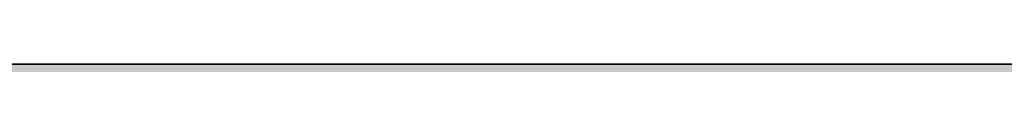
# Model space of a CAD drawing. Units: inches. Extents: x 2091 to 2899, y 967 to 2217.
# Tile 80 of 256: x 2223.2 to 2238.36, y 1099.92 to 1099.92. Entities that reach past the tile are written whole.
import ezdxf

# ---------------------------------------------------------------- set-up
doc = ezdxf.new("R2010")
doc.units = ezdxf.units.IN
doc.layers.add('A-WALL-PATT', color=141, linetype='Continuous', lineweight=13, true_color=0xadddf7)
doc.layers.add('L-SITE-WALL', color=7, linetype='Continuous', lineweight=35)

msp = doc.modelspace()

# ---------------------------------------------------------------- hatches: boundary and pattern name
at = {"layer": 'A-WALL-PATT'}
h = msp.add_hatch(color=256, dxfattribs=at)
h.dxf.hatch_style = 1
h.paths.add_polyline_path([(2212.144, 1941.419), (2387.644, 1941.419), (2387.644, 1824.419), (2392.144, 1824.419), (2392.144, 1941.419), (2609.644, 1941.419), (2609.644, 1825.919), (2614.144, 1825.919), (2614.144, 1941.419), (2794.144, 1941.419), (2794.144, 1928.762), (2803.144, 1928.762), (2803.144, 2050.919), (2203.144, 2050.919), (2203.144, 1900.758), (2212.144, 1900.758)])
h.paths.add_polyline_path([(2212.144, 1945.919), (2212.144, 2041.919), (2794.144, 2041.919), (2794.144, 1945.919), (2402.248, 1945.919), (2401.102, 1945.776), (2398.702, 1945.776)], flags=16)
h.paths.add_polyline_path([(2230.23, 1948.063), (2227.35, 1949.503), (2225.91, 1951.903), (2223.99, 1952.863), (2223.03, 1955.263), (2222.07, 1959.583), (2222.07, 1963.423), (2223.03, 1965.663), (2223.99, 1965.343), (2225.586, 1963.861), (2226.912, 1964.957), (2226.949, 1965.939), (2227.778, 1966.952), (2228.2, 1968.879), (2230.71, 1964.863), (2233.59, 1966.303), (2233.607, 1966.332), (2233.773, 1964.938), (2234.634, 1963.676), (2235.03, 1963.903), (2236.282, 1965.572), (2235.99, 1962.943), (2237.955, 1957.54), (2238.39, 1957.903), (2239.216, 1960.306), (2238.655, 1966.385), (2238.693, 1966.438), (2238.841, 1967.5), (2238.78, 1967.687), (2238.881, 1967.787), (2238.667, 1966.252), (2239.216, 1960.306), (2238.39, 1957.903), (2236.95, 1956.703), (2234.55, 1949.983)], flags=0)
h.paths.add_polyline_path([(2278.012, 1948.063), (2276.496, 1947.873), (2275.85, 1947.689), (2274.652, 1947.103)], flags=0)
h.paths.add_polyline_path([(2269.852, 1955.743), (2268.276, 1956.629), (2270.867, 1956.348), (2269.372, 1958.143), (2268.715, 1959.192), (2270.57, 1958.729), (2268.581, 1961.906), (2270.812, 1960.892), (2270.812, 1963.423), (2271.393, 1964.779), (2270.292, 1966.156), (2271.772, 1965.663), (2272.141, 1966.525), (2273.93, 1965.929), (2275.63, 1968.054), (2276.332, 1966.722), (2276.52, 1966.952), (2276.942, 1968.879), (2277.734, 1967.611), (2278.14, 1969.465), (2279.659, 1967.034), (2280.412, 1966.783), (2280.949, 1967.589), (2281.61, 1967.369), (2282.133, 1968.154), (2282.349, 1966.333), (2282.35, 1966.333), (2283.408, 1968.095), (2283.713, 1965.524), (2284.32, 1964.634), (2284.512, 1964.889), (2284.235, 1965.705), (2284.5, 1967.319), (2284.908, 1965.417), (2285.396, 1966.069), (2285.433, 1966.291), (2285.473, 1966.171), (2286.354, 1967.345), (2286.222, 1966.158), (2287.663, 1968.08), (2287.714, 1968.443), (2288.482, 1969.017), (2288.574, 1968.729), (2288.917, 1969.069), (2288.607, 1966.838), (2288.929, 1963.351), (2288.935, 1963.357), (2288.93, 1963.34), (2289.015, 1962.414), (2290.111, 1963.875), (2290.133, 1963.943), (2290.218, 1964.017), (2290.111, 1963.875), (2289.156, 1960.892), (2288.594, 1959.257), (2288.572, 1959.103), (2289.532, 1960.543), (2290.012, 1962.463), (2290.192, 1962.643), (2289.77, 1959.689), (2286.89, 1957.289), (2284.49, 1950.569), (2283.315, 1950.046), (2283.292, 1949.983), (2280.29, 1948.649), (2281.13, 1948.649), (2282.57, 1948.169), (2283.205, 1948.063), (2278.972, 1948.063), (2276.092, 1949.503), (2274.652, 1951.903), (2272.732, 1952.863)], flags=0)
h.paths.add_polyline_path([(2271.159, 1958.022), (2272.97, 1955.849), (2272.01, 1960.169), (2272.01, 1964.009), (2272.624, 1965.443), (2274.328, 1963.861), (2275.654, 1964.957), (2275.638, 1964.539), (2277.412, 1966.007), (2277.033, 1965.157), (2276.83, 1964.976), (2276.766, 1963.295), (2277.45, 1962.66), (2279.452, 1964.863), (2282.332, 1966.303), (2283.53, 1966.889), (2283.295, 1966.771), (2283.913, 1963.885), (2284.899, 1964.448), (2284.732, 1962.943), (2286.697, 1957.54), (2287.132, 1957.903), (2287.542, 1959.095), (2287.779, 1958.442), (2285.683, 1956.695), (2285.877, 1959.795), (2284.732, 1962.943), (2284.899, 1964.448), (2283.913, 1963.885), (2284.224, 1962.434), (2283.424, 1963.605), (2281.61, 1962.569), (2281.13, 1960.169), (2282.09, 1956.329), (2283.05, 1952.969), (2282.57, 1950.569), (2280.17, 1948.649), (2279.883, 1948.792), (2278.972, 1948.063), (2278.972, 1949.023), (2278.672, 1949.397), (2277.29, 1950.089), (2275.85, 1952.489), (2273.93, 1953.449), (2272.49, 1954.889), (2271.922, 1954.889), (2271.772, 1955.263)], flags=0)
h.paths.add_polyline_path([(2311.994, 1955.743), (2312.063, 1955.674), (2312.055, 1955.709)], flags=0)
h.paths.add_polyline_path([(2331.956, 1963.952), (2333.396, 1965.392), (2331.077, 1963.357), (2330.999, 1963.112)], flags=0)
h.paths.add_polyline_path([(2310.554, 1954.303), (2307.04, 1956.28), (2310.763, 1955.876), (2312.474, 1953.823), (2313.434, 1951.423), (2315.354, 1950.463), (2316.794, 1948.063), (2317.466, 1947.727), (2319.369, 1947.965), (2317.754, 1949.983), (2317.57, 1950.61), (2316.794, 1951.903), (2314.874, 1952.863), (2313.914, 1955.263), (2311.514, 1958.143), (2309.375, 1961.559), (2311.514, 1960.337), (2311.514, 1961.983), (2310.605, 1963.12), (2311.727, 1962.479), (2312.418, 1964.093), (2312.256, 1964.296), (2313.194, 1963.983), (2313.914, 1965.663), (2314.647, 1965.419), (2315.354, 1966.303), (2316.794, 1967.743), (2316.157, 1966.947), (2317.034, 1965.282), (2317.223, 1965.512), (2317.777, 1968.046), (2318.474, 1966.722), (2318.663, 1966.952), (2319.084, 1968.879), (2321.207, 1965.482), (2322.161, 1966.914), (2322.554, 1966.783), (2322.786, 1967.131), (2322.882, 1966.324), (2323.312, 1965.722), (2323.651, 1965.891), (2324.396, 1967.133), (2324.657, 1964.938), (2324.972, 1964.477), (2325.387, 1967.001), (2325.941, 1964.418), (2327.229, 1966.136), (2327.166, 1965.572), (2328.059, 1966.763), (2328.225, 1966.247), (2329.668, 1967.677), (2329.665, 1967.687), (2329.765, 1967.787), (2329.551, 1966.252), (2330.1, 1960.306), (2329.333, 1958.073), (2329.313, 1957.935), (2329.634, 1958.203), (2330.234, 1959.103), (2330.714, 1961.023), (2331.034, 1961.343), (2330.714, 1959.103), (2329.634, 1958.203), (2329.274, 1957.663), (2327.712, 1956.361), (2325.434, 1949.983), (2324.334, 1949.494), (2323.994, 1948.543), (2319.674, 1946.623), (2316.794, 1948.063), (2315.354, 1950.463), (2313.434, 1951.423)], flags=0)
h.paths.add_polyline_path([(2321.336, 1947.952), (2321.114, 1948.063), (2321.114, 1949.023), (2319.194, 1951.423), (2316.794, 1959.583), (2316.663, 1959.583), (2315.354, 1958.143), (2314.394, 1958.143), (2313.148, 1958.709), (2312.954, 1959.583), (2312.954, 1960.892), (2315.834, 1959.583), (2316.663, 1959.583), (2317.315, 1960.299), (2315.03, 1962.421), (2316.356, 1963.517), (2316.372, 1963.952), (2316.47, 1963.861), (2317.796, 1964.957), (2317.755, 1963.89), (2319.175, 1965.157), (2319.498, 1965.881), (2321.114, 1965.343), (2323.236, 1962.372), (2325.686, 1963.773), (2325.543, 1962.481), (2325.199, 1963.494), (2324.479, 1963.082), (2324.926, 1960.994), (2324.078, 1962.236), (2322.415, 1961.286), (2322.074, 1959.583), (2323.034, 1955.743), (2323.994, 1952.383), (2323.514, 1949.983), (2322.143, 1948.886), (2322.074, 1948.543)], flags=0)
h.paths.add_polyline_path([(2320.207, 1963.337), (2320.154, 1963.423), (2320.394, 1963.543)], flags=0)
h.paths.add_polyline_path([(2353.851, 1965.811), (2354.031, 1965.751), (2354.331, 1966.451), (2354.331, 1966.931)], flags=0)
h.paths.add_polyline_path([(2359.021, 1969.026), (2359.098, 1968.902), (2359.234, 1969.52), (2359.234, 1970)], flags=0)
h.paths.add_polyline_path([(2358.257, 1966.682), (2357.984, 1966.348), (2358.211, 1966.146), (2358.41, 1966.39)], flags=0)
h.paths.add_polyline_path([(2357.768, 1966.059), (2357.732, 1965.105), (2357.751, 1965.121), (2357.77, 1965.607), (2357.77, 1966.058)], flags=0)
h.paths.add_polyline_path([(2359.112, 1965.305), (2359.112, 1964.825), (2359.845, 1966.468), (2359.845, 1966.948)], flags=0)
h.paths.add_polyline_path([(2360.224, 1966.621), (2360.699, 1969.363), (2360.699, 1969.843), (2360.211, 1967.026), (2360.211, 1966.643)], flags=0)
h.paths.add_polyline_path([(2363.451, 1967.891), (2363.451, 1968.371), (2362.491, 1966.931), (2362.656, 1966.699)], flags=0)
h.paths.add_polyline_path([(2364.476, 1966.079), (2365.851, 1968.371), (2365.851, 1968.851), (2364.428, 1966.48)], flags=0)
h.paths.add_polyline_path([(2366.314, 1965.853), (2366.367, 1965.696), (2366.803, 1968.346), (2366.803, 1968.826)], flags=0)
h.paths.add_polyline_path([(2367.165, 1965.804), (2367.291, 1966.931), (2367.291, 1967.411), (2367.103, 1965.72)], flags=0)
h.paths.add_polyline_path([(2370.037, 1959.974), (2371.014, 1963.025), (2371.014, 1963.505), (2370.037, 1960.454)], flags=0)
h.paths.add_polyline_path([(2371.611, 1960.211), (2372.571, 1961.651), (2372.571, 1962.131), (2371.803, 1960.979)], flags=0)
h.paths.add_polyline_path([(2350.874, 1956.005), (2351.931, 1955.891), (2354.491, 1953.331), (2353.851, 1954.931), (2351.451, 1957.811), (2347.936, 1963.426), (2347.936, 1963.906), (2351.451, 1958.291), (2353.705, 1955.585), (2352.891, 1959.251), (2352.891, 1959.731), (2352.891, 1961.925), (2356.731, 1959.731), (2358.454, 1961.627), (2354.811, 1965.011), (2355.031, 1965.286), (2358.691, 1961.887), (2361.531, 1965.011), (2364.376, 1966.433), (2364.524, 1965.187), (2365.454, 1963.824), (2365.881, 1964.068), (2365.371, 1966.451), (2365.371, 1966.931), (2366.811, 1960.211), (2366.811, 1959.731), (2366.389, 1952.981), (2367.771, 1956.851), (2368.641, 1957.576), (2366.811, 1962.611), (2366.811, 1963.091), (2368.775, 1957.688), (2369.211, 1958.051), (2370.002, 1960.352), (2369.475, 1966.053), (2369.513, 1966.106), (2369.514, 1966.111), (2369.475, 1966.533), (2369.513, 1966.586), (2369.615, 1967.313), (2369.183, 1968.659), (2369.183, 1969.139), (2369.601, 1967.835), (2369.701, 1967.934), (2369.718, 1968.055), (2370.145, 1968.374), (2369.779, 1968.011), (2369.701, 1967.454), (2370.468, 1968.214), (2369.675, 1967.266), (2369.514, 1966.111), (2370.037, 1960.454), (2370.037, 1959.974), (2369.442, 1958.243), (2370.651, 1959.251), (2371.046, 1962.018), (2371.131, 1962.131), (2370.651, 1958.771), (2367.771, 1956.371), (2365.371, 1949.651), (2362.079, 1948.188), (2363.451, 1947.731), (2361.051, 1947.731), (2360.091, 1947.731), (2357.104, 1947.357), (2360.091, 1948.211), (2358.171, 1949.171), (2356.731, 1951.571), (2354.811, 1952.531), (2351.931, 1955.411)], flags=0)
h.paths.add_polyline_path([(2361.051, 1948.691), (2359.131, 1951.091), (2356.731, 1959.251), (2355.771, 1959.251), (2352.891, 1960.56), (2352.891, 1961.445), (2355.891, 1959.731), (2356.731, 1959.731), (2356.837, 1959.368), (2361.531, 1964.531), (2363.248, 1965.389), (2364.925, 1963.042), (2362.491, 1961.651), (2362.064, 1959.517), (2362.971, 1955.891), (2363.931, 1952.531), (2363.931, 1952.051), (2363.451, 1949.651), (2361.051, 1947.731)], flags=0)
h.paths.add_polyline_path([(2359.131, 1951.571), (2359.291, 1951.371), (2361.051, 1954.451), (2361.051, 1954.931)], flags=0)
h.paths.add_polyline_path([(2357.22, 1966.546), (2356.793, 1968.815), (2356.793, 1969.295), (2357.22, 1967.026)], flags=0)
h.paths.add_polyline_path([(2361.051, 1954.451), (2361.531, 1958.771), (2361.531, 1959.251), (2361.051, 1954.931)], flags=0)
h.paths.add_polyline_path([(2402.548, 1948.486), (2402.302, 1948.416), (2402.59, 1948.416)], flags=0)
h.paths.add_polyline_path([(2394.142, 1956.096), (2395.685, 1954.553), (2396.72, 1953.971), (2396.062, 1955.616), (2395.241, 1956.601), (2395.879, 1956.442), (2395.102, 1959.936), (2395.102, 1963.776), (2396.062, 1966.016), (2397.022, 1965.696), (2398.618, 1964.214), (2399.944, 1965.31), (2399.981, 1966.292), (2400.811, 1967.305), (2401.232, 1969.232), (2403.538, 1965.543), (2403.942, 1967.389), (2404.702, 1967.136), (2405.46, 1966.075), (2406.622, 1966.656), (2406.64, 1966.685), (2406.805, 1965.291), (2406.926, 1965.115), (2407.342, 1964.976), (2407.874, 1965.774), (2408.169, 1964.398), (2409.315, 1965.925), (2409.217, 1965.051), (2409.445, 1963.131), (2410.306, 1961.87), (2410.702, 1962.096), (2411.442, 1963.082), (2411.165, 1963.898), (2411.616, 1966.64), (2411.725, 1966.791), (2411.873, 1967.853), (2411.813, 1968.041), (2411.913, 1968.14), (2411.699, 1966.605), (2412.248, 1960.659), (2413.225, 1963.71), (2414.378, 1964.721), (2414.513, 1965.693), (2414.453, 1965.881), (2414.553, 1965.98), (2414.378, 1964.721), (2414.52, 1964.846), (2414.365, 1964.631), (2414.339, 1964.445), (2414.888, 1958.499), (2414.062, 1956.096), (2412.622, 1954.896), (2410.171, 1948.033), (2410.017, 1948.084), (2405.902, 1946.256), (2405.902, 1947.216), (2405.204, 1948.089), (2404.222, 1948.416), (2403.262, 1948.416), (2400.382, 1949.856), (2399.662, 1951.056), (2397.982, 1952.736), (2397.022, 1953.216), (2395.685, 1954.553), (2392.657, 1956.257)], flags=0)
h.paths.add_polyline_path([(2409.086, 1964.407), (2409.13, 1964.276), (2409.262, 1964.496)], flags=0)
h.paths.add_polyline_path([(2397.742, 1961.616), (2398.702, 1963.856), (2399.662, 1963.536), (2401.427, 1965.741), (2401.791, 1966.559), (2402.071, 1965.071), (2402.836, 1964.393), (2403.262, 1964.915), (2403.338, 1964.771), (2402.616, 1963.976), (2402.499, 1960.902), (2403.543, 1959.932), (2404.413, 1960.89), (2404.702, 1962.336), (2407.916, 1964.172), (2409.52, 1961.927), (2410.987, 1957.893), (2411.422, 1958.256), (2412.048, 1960.076), (2412.41, 1959.079), (2411.676, 1958.467), (2411.662, 1958.256), (2411.626, 1958.426), (2409.982, 1957.056), (2407.582, 1950.336), (2403.262, 1948.416), (2403.262, 1949.376), (2401.342, 1951.776), (2399.417, 1958.324), (2397.742, 1959.085), (2397.742, 1959.97), (2397.102, 1960.336), (2397.742, 1960.045)], flags=0)
h.paths.add_polyline_path([(2405.902, 1952.976), (2405.95, 1953.408), (2406.017, 1953.176)], flags=0)
h.paths.add_polyline_path([(2449.818, 1967.114), (2449.752, 1967.136), (2449.794, 1967.078)], flags=0)
h.paths.add_polyline_path([(2451.698, 1966.618), (2451.741, 1966.69), (2451.692, 1966.666)], flags=0)
h.paths.add_polyline_path([(2454.344, 1965.738), (2455.752, 1967.616), (2455.992, 1968.096), (2454.364, 1965.925)], flags=0)
h.paths.add_polyline_path([(2457.547, 1968.864), (2457.787, 1969.344), (2457.054, 1968.796), (2457.008, 1968.46)], flags=0)
h.paths.add_polyline_path([(2456.922, 1967.857), (2456.802, 1968.229), (2456.723, 1967.66)], flags=0)
h.paths.add_polyline_path([(2457.302, 1967.377), (2457.542, 1967.857), (2456.81, 1966.84), (2456.741, 1966.7), (2456.749, 1966.608)], flags=0)
h.paths.add_polyline_path([(2458.275, 1963.71), (2458.155, 1963.335), (2460.354, 1965.265), (2460.594, 1965.745)], flags=0)
h.paths.add_polyline_path([(2458.392, 1962.816), (2458.364, 1962.618), (2459.592, 1964.256), (2459.832, 1964.736)], flags=0)
h.paths.add_polyline_path([(2459.352, 1962.816), (2459.272, 1962.496), (2460.072, 1963.296), (2460.312, 1963.776)], flags=0)
h.paths.add_polyline_path([(2458.68, 1960.608), (2458.632, 1960.416), (2459.592, 1961.856), (2459.832, 1962.336)], flags=0)
h.paths.add_polyline_path([(2437.838, 1956.243), (2439.192, 1956.096), (2441.352, 1953.936), (2440.872, 1955.136), (2438.472, 1958.016), (2438.072, 1958.656), (2438.712, 1958.496), (2440.64, 1956.183), (2439.912, 1959.456), (2439.912, 1963.296), (2441.352, 1966.656), (2441.592, 1967.136), (2441.112, 1966.016), (2442.072, 1965.696), (2443.989, 1968.092), (2444.241, 1966.751), (2444.917, 1966.152), (2445.677, 1967.08), (2446.255, 1969.725), (2446.495, 1970.205), (2446.282, 1969.232), (2447.363, 1967.503), (2447.72, 1969.568), (2447.96, 1970.048), (2447.485, 1967.307), (2448.792, 1965.216), (2448.472, 1964.864), (2448.552, 1964.736), (2451.452, 1966.186), (2451.615, 1964.811), (2452.308, 1963.796), (2453.235, 1964.326), (2454.072, 1960.416), (2453.629, 1953.318), (2454.792, 1956.576), (2455.032, 1957.056), (2455.719, 1957.628), (2453.832, 1962.816), (2453.941, 1963.794), (2453.335, 1965.578), (2453.824, 1968.551), (2454.064, 1969.031), (2453.575, 1966.058), (2454.04, 1964.688), (2453.832, 1962.816), (2455.719, 1957.628), (2456.367, 1958.168), (2457.058, 1960.179), (2457.298, 1960.659), (2456.472, 1958.256), (2457.718, 1959.294), (2457.672, 1958.976), (2454.89, 1956.657), (2453.614, 1953.085), (2453.592, 1952.736), (2453.352, 1952.256), (2453.36, 1952.372), (2452.632, 1950.336), (2452.392, 1949.856), (2449.204, 1948.439), (2450.712, 1947.936), (2448.072, 1947.936), (2447.112, 1947.936), (2444.552, 1947.616), (2447.2, 1948.372), (2445.192, 1949.376), (2443.752, 1951.776), (2441.832, 1952.736), (2438.952, 1955.616)], flags=0)
h.paths.add_polyline_path([(2443.992, 1959.936), (2444.04, 1959.773), (2444.122, 1959.862)], flags=0)
h.paths.add_polyline_path([(2442.912, 1959.936), (2443.032, 1959.936), (2442.446, 1960.202)], flags=0)
h.paths.add_polyline_path([(2444.983, 1965.02), (2445.279, 1965.265), (2445.519, 1965.745), (2444.994, 1965.31)], flags=0)
h.paths.add_polyline_path([(2446.133, 1965.03), (2446.33, 1965.471), (2444.97, 1964.258), (2444.73, 1963.778)], flags=0)
h.paths.add_polyline_path([(2442.792, 1959.456), (2443.752, 1959.456), (2446.152, 1951.296), (2446.412, 1951.751), (2446.392, 1951.776), (2448.081, 1954.73), (2448.552, 1958.976), (2441.832, 1965.216), (2442.155, 1965.619), (2448.792, 1959.456), (2448.312, 1955.136), (2448.072, 1954.656), (2446.412, 1951.751), (2448.312, 1949.376), (2448.312, 1948.416), (2450.541, 1950.199), (2450.952, 1952.256), (2449.992, 1955.616), (2449.032, 1959.456), (2449.512, 1961.856), (2449.752, 1962.336), (2449.675, 1961.949), (2452.995, 1963.846), (2453.064, 1963.519), (2452.885, 1963.783), (2449.675, 1961.949), (2449.272, 1959.936), (2450.232, 1956.096), (2451.192, 1952.736), (2450.712, 1950.336), (2450.472, 1949.856), (2448.072, 1947.936), (2448.072, 1948.536), (2445.432, 1949.856), (2443.992, 1952.256), (2442.072, 1953.216), (2441.112, 1955.616), (2440.152, 1959.936), (2440.152, 1960.656)], flags=0)
h.paths.add_polyline_path([(2456.692, 1966.986), (2457.608, 1968.081), (2457.848, 1968.561), (2456.932, 1967.466)], flags=0)
h.paths.add_polyline_path([(2489.897, 1966.58), (2489.943, 1966.189), (2490.747, 1967.53), (2491.319, 1968.951)], flags=0)
h.paths.add_polyline_path([(2473.562, 1956.407), (2477.14, 1956.019), (2476.955, 1956.241), (2475.108, 1957.28), (2476.347, 1956.97), (2475.187, 1958.824), (2476.919, 1958.391), (2475.412, 1960.799), (2477.787, 1959.719), (2477.787, 1962.25), (2477.637, 1962.438), (2477.823, 1962.332), (2478.359, 1963.584), (2478.359, 1963.671), (2477.324, 1964.965), (2478.715, 1964.501), (2479.319, 1965.911), (2480.279, 1965.591), (2481.784, 1967.472), (2482.116, 1965.705), (2482.881, 1965.028), (2483.209, 1965.429), (2483.22, 1965.715), (2483.076, 1965.989), (2483.712, 1966.766), (2484.13, 1968.679), (2484.702, 1970.1), (2484.489, 1969.127), (2486.503, 1965.905), (2487.387, 1965.61), (2488.153, 1966.759), (2488.717, 1965.97), (2489.2, 1966.212), (2489.331, 1965.111), (2490.394, 1963.622), (2490.661, 1963.775), (2490.494, 1964.554), (2490.923, 1963.925), (2491.319, 1964.151), (2491.333, 1964.17), (2491.21, 1964.532), (2491.282, 1964.966), (2491.426, 1964.293), (2494.076, 1967.828), (2494.498, 1966.515), (2494.598, 1966.614), (2494.689, 1967.27), (2495.107, 1967.582), (2495.13, 1967.748), (2495.07, 1967.936), (2495.17, 1968.035), (2495.032, 1967.044), (2495.754, 1967.759), (2494.982, 1966.686), (2494.956, 1966.5), (2495.479, 1960.837), (2495.91, 1962.184), (2496.482, 1963.605), (2496.073, 1962.327), (2496.769, 1962.938), (2496.599, 1962.711), (2496.119, 1959.351), (2496.733, 1960.272), (2496.987, 1961.29), (2497.559, 1962.711), (2497.079, 1960.791), (2496.507, 1959.37), (2495.547, 1957.93), (2492.759, 1955.606), (2490.839, 1950.231), (2490.267, 1948.81), (2485.947, 1946.89), (2483.067, 1948.33), (2481.627, 1950.73), (2479.707, 1951.69), (2476.827, 1954.57)], flags=0)
h.paths.add_polyline_path([(2485.577, 1948.313), (2485.559, 1948.311), (2485.579, 1948.311)], flags=0)
h.paths.add_polyline_path([(2478.645, 1954.551), (2478.109, 1956.963), (2479.319, 1955.511), (2480.279, 1953.111), (2482.199, 1952.151), (2483.639, 1949.751), (2486.519, 1948.311), (2486.519, 1949.271), (2484.739, 1951.496), (2484.027, 1950.25), (2481.627, 1958.41), (2482.375, 1959.233), (2482.199, 1959.831), (2483.198, 1960.929), (2479.707, 1964.17), (2480.603, 1965.29), (2481.875, 1964.109), (2482.666, 1964.764), (2482.615, 1963.422), (2482.989, 1963.075), (2484.008, 1963.984), (2484.684, 1965.498), (2484.58, 1965.405), (2485.357, 1967.147), (2485.121, 1965.781), (2486.427, 1963.69), (2488.145, 1964.549), (2489.822, 1962.202), (2490.747, 1962.73), (2492, 1964.4), (2492.076, 1965.087), (2492.213, 1964.684), (2492.485, 1965.047), (2492.279, 1963.191), (2494.244, 1957.788), (2494.563, 1958.054), (2494.933, 1959.133), (2495.505, 1960.554), (2494.679, 1958.151), (2494.107, 1956.73), (2494.563, 1958.054), (2493.409, 1957.092), (2491.707, 1961.77), (2492, 1964.4), (2490.747, 1962.73), (2487.712, 1960.996), (2487.479, 1959.831), (2488.439, 1955.991), (2489.399, 1952.631), (2488.919, 1950.231), (2488.577, 1949.957), (2488.347, 1948.81), (2487.652, 1948.254), (2487.479, 1948.311), (2486.519, 1948.311), (2483.639, 1949.751), (2482.199, 1952.151), (2480.279, 1953.111), (2478.839, 1954.551)], flags=0)
h.paths.add_polyline_path([(2526.648, 1966.988), (2526.517, 1967.031), (2526.6, 1966.915)], flags=0)
h.paths.add_polyline_path([(2528.471, 1966.447), (2528.574, 1966.62), (2528.457, 1966.561)], flags=0)
h.paths.add_polyline_path([(2534.133, 1967.496), (2534.157, 1967.543), (2534.06, 1967.408)], flags=0)
h.paths.add_polyline_path([(2536.162, 1964.051), (2535.157, 1962.711), (2535.101, 1962.316), (2536.117, 1963.671), (2536.421, 1964.278)], flags=0)
h.paths.add_polyline_path([(2535.157, 1959.831), (2536.117, 1961.271), (2536.597, 1962.231), (2535.253, 1960.215)], flags=0)
h.paths.add_polyline_path([(2513.249, 1956.285), (2516.221, 1955.963), (2514.997, 1957.431), (2514.196, 1958.712), (2515.477, 1958.391), (2516.932, 1956.646), (2516.437, 1958.871), (2516.437, 1962.711), (2516.873, 1963.727), (2515.346, 1965.635), (2517.397, 1964.951), (2517.877, 1966.071), (2518.357, 1967.031), (2517.877, 1965.911), (2518.837, 1965.591), (2520.487, 1967.653), (2520.766, 1966.166), (2521.53, 1965.489), (2521.781, 1965.795), (2521.801, 1966.307), (2521.478, 1966.921), (2521.246, 1967.126), (2521.178, 1967.491), (2521.478, 1966.921), (2522.01, 1966.449), (2522.257, 1966.75), (2522.78, 1969.14), (2523.26, 1970.1), (2523.047, 1969.127), (2524.673, 1966.526), (2526.037, 1966.071), (2526.795, 1965.01), (2527.977, 1965.601), (2528.14, 1964.227), (2528.665, 1963.458), (2529.389, 1963.872), (2529.33, 1964.147), (2529.481, 1963.925), (2529.877, 1964.151), (2529.984, 1964.293), (2529.789, 1965.203), (2530.062, 1964.398), (2532.802, 1968.051), (2533.148, 1966.976), (2533.248, 1967.075), (2533.339, 1967.731), (2533.673, 1967.98), (2533.728, 1968.035), (2533.514, 1966.5), (2534.025, 1960.972), (2534.56, 1962.645), (2535.04, 1963.605), (2534.063, 1960.554), (2533.237, 1958.151), (2534.288, 1959.027), (2534.197, 1958.391), (2531.513, 1956.154), (2529.397, 1950.231), (2528.917, 1949.271), (2526.449, 1948.174), (2527.477, 1947.831), (2530.357, 1947.351), (2524.597, 1947.351), (2521.717, 1948.791), (2520.277, 1951.191), (2518.357, 1952.151), (2515.477, 1955.031)], flags=0)
h.paths.add_polyline_path([(2523.935, 1967.19), (2523.62, 1966.484), (2523.77, 1966.242)], flags=0)
h.paths.add_polyline_path([(2518.837, 1953.111), (2517.877, 1955.511), (2516.885, 1959.977), (2516.917, 1959.962), (2516.917, 1962.025), (2520.757, 1959.831), (2522.025, 1961.226), (2518.357, 1964.631), (2519.003, 1965.438), (2520.433, 1964.109), (2521.301, 1964.827), (2521.245, 1963.355), (2525.638, 1959.276), (2526.037, 1961.271), (2529.397, 1963.191), (2530.65, 1964.861), (2530.665, 1964.998), (2530.692, 1964.917), (2531.088, 1965.445), (2530.946, 1964.169), (2530.692, 1964.917), (2529.397, 1963.191), (2526.363, 1961.457), (2526.037, 1959.831), (2526.997, 1955.991), (2527.957, 1952.631), (2527.477, 1950.231), (2527.134, 1949.957), (2526.974, 1949.154), (2526.697, 1949.031), (2524.597, 1947.351), (2524.597, 1948.311), (2524.277, 1948.711), (2522.197, 1949.751), (2520.757, 1952.151)], flags=0)
h.paths.add_polyline_path([(2520.277, 1958.871), (2520.853, 1959.505), (2523.157, 1951.671), (2524.614, 1954.22), (2524.597, 1954.071), (2522.677, 1950.711)], flags=0)
h.paths.add_polyline_path([(2559.371, 1966.311), (2559.398, 1966.325), (2559.402, 1966.345)], flags=0)
h.paths.add_polyline_path([(2549.771, 1957.191), (2552.651, 1954.311), (2552.134, 1955.603), (2550.611, 1957.431), (2547.096, 1963.046), (2545.776, 1965.206), (2549.291, 1959.591), (2551.691, 1956.711), (2550.793, 1960.752), (2550.731, 1960.78), (2550.731, 1964.871), (2551.691, 1967.111), (2552.651, 1966.791), (2554.247, 1965.309), (2555.034, 1965.96), (2555.582, 1966.645), (2555.61, 1967.387), (2556.439, 1968.401), (2556.861, 1970.327), (2559.371, 1966.311), (2560.691, 1964.151), (2562.409, 1965.01), (2561.651, 1966.071), (2560.331, 1968.231), (2561.758, 1966.233), (2562.347, 1967.116), (2562.434, 1966.387), (2563.128, 1965.37), (2563.571, 1965.591), (2563.588, 1965.62), (2563.363, 1967.524), (2563.722, 1965.844), (2565.06, 1968.073), (2564.733, 1965.129), (2565.118, 1963.333), (2567.445, 1966.436), (2567.316, 1967.833), (2567.354, 1967.886), (2567.502, 1968.948), (2567.441, 1969.136), (2567.542, 1969.235), (2567.328, 1967.7), (2567.877, 1961.754), (2568.747, 1964.47), (2568.636, 1965.673), (2568.674, 1965.726), (2568.822, 1966.788), (2568.761, 1966.976), (2568.862, 1967.075), (2568.648, 1965.54), (2568.726, 1964.693), (2568.854, 1964.805), (2568.747, 1964.47), (2568.817, 1963.706), (2568.971, 1963.911), (2568.866, 1963.177), (2569.197, 1959.594), (2568.371, 1957.191), (2566.931, 1955.991), (2564.62, 1949.521), (2564.651, 1949.511), (2564.617, 1949.511), (2564.531, 1949.271), (2560.211, 1947.351), (2557.331, 1948.791), (2556.045, 1950.934), (2556.011, 1950.951), (2555.857, 1951.208), (2553.971, 1952.151), (2551.091, 1955.031), (2546.65, 1957.53)], flags=0)
h.paths.add_polyline_path([(2567.026, 1959.33), (2567.035, 1959.305), (2567.051, 1959.351)], flags=0)
h.paths.add_polyline_path([(2551.968, 1962.518), (2553.011, 1964.951), (2553.971, 1964.631), (2555.567, 1963.149), (2556.893, 1964.246), (2556.93, 1965.227), (2557.144, 1965.489), (2556.42, 1966.131), (2556.391, 1966.105), (2556.38, 1966.166), (2556.42, 1966.131), (2556.952, 1966.605), (2557.092, 1966.919), (2557.571, 1966.01), (2557.759, 1966.241), (2557.418, 1964.68), (2556.893, 1964.246), (2556.807, 1961.998), (2560.691, 1958.391), (2560.636, 1957.893), (2560.811, 1957.191), (2561.771, 1953.831), (2561.291, 1951.431), (2559.11, 1949.687), (2559.156, 1949.629), (2563.027, 1951.349), (2562.611, 1949.271), (2560.211, 1947.351), (2560.211, 1948.311), (2559.251, 1949.511), (2558.891, 1949.511), (2558.891, 1949.961), (2558.291, 1950.711), (2558.054, 1951.518), (2556.971, 1952.871), (2555.068, 1959.341), (2552.051, 1961.065), (2552.051, 1962.471)], flags=0)
h.paths.add_polyline_path([(2588.33, 1958.391), (2588.61, 1958.111), (2588.553, 1958.367)], flags=0)
h.paths.add_polyline_path([(2594.745, 1950.493), (2593.958, 1953.172), (2593.13, 1954.551), (2591.21, 1955.511), (2590.25, 1957.911), (2588.309, 1960.24), (2586.177, 1961.209), (2587.85, 1960.791), (2587.253, 1961.744), (2588.441, 1961.065), (2588.441, 1962.656), (2588.422, 1962.665), (2588.441, 1962.711), (2586.914, 1964.62), (2588.877, 1963.728), (2589.29, 1964.692), (2589.29, 1966.071), (2590.25, 1968.311), (2591.21, 1967.991), (2592.806, 1966.509), (2594.132, 1967.606), (2594.169, 1968.587), (2594.999, 1969.601), (2595.42, 1971.527), (2597.93, 1967.511), (2600.81, 1968.951), (2600.827, 1968.98), (2600.993, 1967.587), (2601.854, 1966.325), (2602.107, 1966.47), (2602.236, 1967.255), (2602.357, 1966.693), (2603.502, 1968.221), (2603.21, 1965.591), (2605.175, 1960.188), (2605.507, 1960.465), (2605.026, 1965.673), (2605.064, 1965.726), (2605.212, 1966.788), (2605.152, 1966.976), (2605.252, 1967.075), (2605.343, 1967.731), (2605.953, 1968.187), (2605.875, 1969.033), (2605.913, 1969.086), (2606.061, 1970.148), (2606, 1970.336), (2606.101, 1970.435), (2605.887, 1968.9), (2606.436, 1962.954), (2605.61, 1960.551), (2605.997, 1960.874), (2606.564, 1962.645), (2608.241, 1964.117), (2608.01, 1963.191), (2607.05, 1961.751), (2606.631, 1961.402), (2606.201, 1958.391), (2603.321, 1955.991), (2600.921, 1949.271), (2596.601, 1947.351), (2593.721, 1948.791), (2592.857, 1950.231), (2592.65, 1950.231)], flags=0)
h.paths.add_polyline_path([(2596.601, 1947.351), (2596.601, 1948.311), (2594.681, 1950.711), (2596.155, 1953.29), (2595.53, 1954.071), (2593.199, 1961.996), (2592.651, 1962.505), (2591.78, 1963.003), (2593.283, 1964.246), (2593.32, 1965.227), (2594.15, 1966.241), (2594.571, 1968.167), (2596.183, 1965.589), (2596.951, 1966.435), (2598.041, 1966.071), (2598.799, 1965.01), (2599.961, 1965.591), (2599.979, 1965.62), (2600.144, 1964.227), (2601.005, 1962.965), (2601.401, 1963.191), (2602.653, 1964.861), (2602.361, 1962.231), (2603.793, 1958.295), (2601.978, 1953.212), (2601.946, 1952.709), (2599.469, 1951.608), (2599.001, 1949.271)], flags=0)
h.paths.add_polyline_path([(2597.561, 1958.871), (2597.671, 1959.419), (2597.595, 1958.736)], flags=0)
h.paths.add_polyline_path([(2623.666, 1961.254), (2625.519, 1960.791), (2624.966, 1961.676), (2627.199, 1960.66), (2627.199, 1961.151), (2626.959, 1962.231), (2626.959, 1963.491), (2625.582, 1965.212), (2626.959, 1964.425), (2626.959, 1965.831), (2626.869, 1965.861), (2627.919, 1968.311), (2628.879, 1967.991), (2630.475, 1966.509), (2631.801, 1967.606), (2631.838, 1968.587), (2632.668, 1969.601), (2633.089, 1971.527), (2635.599, 1967.511), (2638.479, 1968.951), (2638.497, 1968.98), (2638.662, 1967.587), (2639.176, 1966.833), (2639.78, 1967.84), (2640.026, 1966.693), (2641.171, 1968.221), (2640.879, 1965.591), (2641.114, 1964.945), (2641.411, 1965.341), (2641.308, 1964.412), (2642.844, 1960.188), (2643.279, 1960.551), (2644.085, 1962.895), (2643.784, 1966.153), (2643.807, 1966.185), (2643.601, 1968.418), (2643.523, 1968.661), (2643.73, 1970.148), (2643.67, 1970.336), (2643.77, 1970.435), (2643.556, 1968.9), (2643.601, 1968.418), (2643.91, 1967.456), (2644.01, 1967.555), (2643.812, 1966.132), (2644.105, 1962.954), (2644.239, 1961.351), (2644.719, 1961.751), (2645.033, 1962.222), (2645.322, 1963.125), (2646.076, 1963.787), (2645.033, 1962.222), (2644.345, 1960.074), (2643.519, 1957.671), (2642.079, 1956.471), (2639.72, 1949.864), (2639.876, 1949.838), (2635.359, 1947.831), (2632.479, 1949.271), (2631.039, 1951.671), (2629.119, 1952.631), (2628.159, 1955.031), (2625.759, 1957.911)], flags=0)
h.paths.add_polyline_path([(2627.816, 1956.574), (2627.374, 1958.566), (2626.376, 1959.763), (2627.199, 1959.351), (2627.374, 1958.566), (2627.919, 1957.911), (2628.879, 1955.511), (2630.799, 1954.551), (2632.239, 1952.151), (2633.315, 1951.613), (2631.039, 1959.351), (2631.498, 1959.856), (2630.799, 1962.231), (2631.45, 1962.947), (2630.715, 1963.629), (2632.041, 1964.726), (2632.078, 1965.707), (2632.292, 1965.969), (2631.705, 1966.489), (2633.136, 1967.766), (2633.329, 1968.647), (2634.675, 1966.494), (2635.208, 1967.081), (2636.799, 1966.551), (2637.676, 1967.867), (2638.994, 1966.022), (2639.705, 1966.429), (2641.119, 1959.831), (2640.93, 1956.806), (2639.439, 1952.631), (2638.227, 1952.093), (2637.759, 1949.751), (2635.359, 1947.831), (2635.359, 1948.791), (2633.439, 1951.191), (2633.315, 1951.613), (2632.239, 1952.151), (2630.799, 1954.551), (2628.879, 1955.511)], flags=0)
h.paths.add_polyline_path([(2637.759, 1953.831), (2637.279, 1955.511), (2636.319, 1959.351), (2636.799, 1961.751), (2639.234, 1963.142), (2637.557, 1965.49), (2638.739, 1966.081), (2638.902, 1964.707), (2639.763, 1963.445), (2636.799, 1961.751), (2636.532, 1960.418), (2637.039, 1958.391), (2637.999, 1955.031)], flags=0)
h.paths.add_polyline_path([(2668.567, 1951.431), (2667.607, 1953.831), (2665.207, 1956.711), (2662.294, 1961.365), (2665.447, 1959.591), (2666.647, 1958.391), (2666.647, 1959.975), (2666.058, 1960.682), (2666.647, 1960.345), (2666.647, 1961.991), (2666.7, 1962.114), (2666.407, 1963.431), (2666.407, 1967.271), (2667.367, 1969.511), (2668.327, 1969.191), (2669.923, 1967.709), (2671.249, 1968.806), (2671.286, 1969.787), (2672.116, 1970.801), (2672.537, 1972.727), (2675.047, 1968.711), (2677.927, 1970.151), (2677.945, 1970.18), (2678.11, 1968.787), (2678.971, 1967.525), (2679.367, 1967.751), (2680.62, 1969.421), (2680.327, 1966.791), (2682.292, 1961.388), (2682.727, 1961.751), (2683.358, 1963.587), (2683.232, 1964.953), (2683.27, 1965.006), (2683.393, 1965.889), (2683.36, 1966.249), (2683.358, 1966.256), (2683.359, 1966.257), (2682.992, 1970.233), (2683.03, 1970.286), (2683.178, 1971.348), (2683.118, 1971.536), (2683.218, 1971.635), (2683.004, 1970.1), (2683.359, 1966.257), (2683.458, 1966.355), (2683.393, 1965.889), (2683.414, 1965.665), (2684.424, 1966.872), (2683.553, 1964.154), (2683.358, 1963.587), (2683.793, 1958.874), (2682.967, 1956.471), (2681.527, 1955.271), (2680.109, 1951.3), (2680.085, 1950.912), (2679.977, 1950.93), (2679.127, 1948.551), (2674.807, 1946.631), (2671.927, 1948.071), (2670.487, 1950.471)], flags=0)
h.paths.add_polyline_path([(2671.936, 1953.227), (2671.687, 1953.351), (2670.247, 1955.751), (2668.327, 1956.711), (2667.357, 1959.138), (2669.527, 1958.151), (2670.487, 1958.151), (2671.479, 1959.242), (2670.684, 1961.945), (2668.89, 1963.612), (2667.307, 1964.331), (2668.567, 1963.911), (2668.831, 1964.241), (2670.247, 1963.431), (2672.422, 1965.823), (2672.777, 1967.447), (2673.234, 1966.716), (2674.412, 1968.012), (2673.981, 1965.522), (2675.287, 1963.431), (2675.554, 1963.564), (2675.932, 1965.456), (2676.247, 1965.351), (2677.005, 1964.29), (2678.167, 1964.871), (2679.607, 1967.271), (2680.327, 1963.911), (2680.307, 1963.577), (2680.347, 1963.458), (2680.86, 1964.141), (2680.567, 1961.511), (2681.104, 1960.037), (2678.887, 1953.831), (2677.092, 1953.033), (2677.687, 1950.951), (2677.207, 1948.551), (2674.807, 1946.631), (2674.807, 1947.591), (2672.887, 1949.991)], flags=0)
h.paths.add_polyline_path([(2673.985, 1951.911), (2674.567, 1952.931), (2674.567, 1951.911), (2676.967, 1953.831), (2677.447, 1956.231), (2676.487, 1959.591), (2676.247, 1960.551), (2679.73, 1962.541), (2680.059, 1961.002), (2679.211, 1962.245), (2676.247, 1960.551), (2676.487, 1959.591), (2677.447, 1956.231), (2676.967, 1953.831), (2674.567, 1951.911)], flags=0)
h.paths.add_polyline_path([(2707.479, 1952.815), (2706.519, 1955.215), (2705.559, 1959.535), (2705.559, 1963.375), (2706.519, 1965.615), (2707.479, 1965.295), (2709.075, 1963.813), (2710.401, 1964.909), (2710.438, 1965.891), (2711.268, 1966.904), (2711.689, 1968.831), (2714.199, 1964.815), (2717.079, 1966.255), (2717.097, 1966.284), (2717.262, 1964.89), (2718.123, 1963.628), (2718.519, 1963.855), (2719.771, 1965.524), (2719.479, 1962.895), (2721.444, 1957.492), (2721.879, 1957.855), (2722.705, 1960.258), (2722.144, 1966.337), (2722.182, 1966.39), (2722.33, 1967.452), (2722.27, 1967.639), (2722.37, 1967.739), (2722.156, 1966.204), (2722.705, 1960.258), (2721.879, 1957.855), (2720.439, 1956.655), (2718.039, 1949.935), (2713.719, 1948.015), (2710.839, 1949.455), (2709.399, 1951.855)], flags=0)
h.paths.add_polyline_path([(2749.301, 1952.815), (2748.341, 1955.215), (2747.381, 1959.535), (2747.381, 1963.375), (2748.341, 1965.615), (2749.301, 1965.295), (2750.897, 1963.813), (2752.223, 1964.909), (2752.26, 1965.891), (2753.09, 1966.904), (2753.511, 1968.831), (2756.021, 1964.815), (2758.901, 1966.255), (2758.919, 1966.284), (2759.084, 1964.89), (2759.945, 1963.628), (2760.341, 1963.855), (2761.593, 1965.524), (2761.301, 1962.895), (2763.266, 1957.492), (2763.701, 1957.855), (2764.527, 1960.258), (2763.966, 1966.337), (2764.004, 1966.39), (2764.152, 1967.452), (2764.092, 1967.639), (2764.192, 1967.739), (2763.978, 1966.204), (2764.527, 1960.258), (2763.701, 1957.855), (2762.261, 1956.655), (2759.861, 1949.935), (2755.541, 1948.015), (2752.661, 1949.455), (2751.221, 1951.855)], flags=0)
h.paths.add_polyline_path([(2212.144, 1819.935), (2203.144, 1819.935), (2203.144, 1739.98), (2212.144, 1739.98), (2212.144, 1780.919), (2392.144, 1780.919), (2392.144, 1783.919), (2212.144, 1783.919)])
h.paths.add_polyline_path([(2803.144, 1847.939), (2794.144, 1847.939), (2794.144, 1785.419), (2609.644, 1785.419), (2493.876, 1785.419), (2493.876, 1780.919), (2609.644, 1780.919), (2794.144, 1780.919), (2794.144, 1696.919), (2609.376, 1696.919), (2609.376, 1742.919), (2604.876, 1742.919), (2604.876, 1644.419), (2609.376, 1644.419), (2609.376, 1692.419), (2794.144, 1692.419), (2794.144, 1668.165), (2803.144, 1668.165)])
h.paths.add_polyline_path([(2392.144, 1740.419), (2387.644, 1740.419), (2387.644, 1629.419), (2212.144, 1629.419), (2212.144, 1659.156), (2203.144, 1659.156), (2203.144, 1494.089), (2212.144, 1494.089), (2212.144, 1627.919), (2392.144, 1627.919)])
h.paths.add_polyline_path([(2457.876, 1780.919), (2453.376, 1780.919), (2453.376, 1644.419), (2568.876, 1644.419), (2568.876, 1648.919), (2457.876, 1648.919)])
h.paths.add_polyline_path([(2545.144, 1591.919), (2540.644, 1591.919), (2540.644, 1567.919), (2468.644, 1567.919), (2468.644, 1627.919), (2509.144, 1627.919), (2509.144, 1632.419), (2464.144, 1632.419), (2464.144, 1563.419), (2545.144, 1563.419)])
h.paths.add_polyline_path([(2268.644, 1555.919), (2212.144, 1555.919), (2212.144, 1551.419), (2268.644, 1551.419)], flags=17)
h.paths.add_polyline_path([(2212.144, 1413.266), (2203.144, 1413.266), (2203.144, 1233.07), (2212.144, 1233.07)])
h.paths.add_polyline_path([(2267.644, 1351.919), (2212.144, 1351.919), (2212.144, 1347.419), (2267.644, 1347.419)], flags=17)
h.paths.add_polyline_path([(2456.644, 1489.419), (2452.144, 1489.419), (2452.144, 1351.919), (2312.644, 1351.919), (2312.644, 1347.419), (2456.644, 1347.419)])
h.paths.add_polyline_path([(2472.37, 1455.419), (2467.87, 1455.419), (2467.87, 1347.419), (2472.37, 1347.419)])
h.paths.add_polyline_path([(2794.144, 1351.919), (2543.37, 1351.919), (2543.37, 1347.419), (2794.144, 1347.419)], flags=17)
h.paths.add_polyline_path([(2312.644, 1347.419), (2308.144, 1347.419), (2308.144, 1302.162), (2308.342, 1302.164), (2308.144, 1298.169), (2308.144, 1275.419), (2212.144, 1275.419), (2212.144, 1270.919), (2312.644, 1270.919)], flags=17)
h.paths.add_polyline_path([(2212.144, 1152.247), (2203.144, 1152.247), (2203.144, 1090.919), (2803.144, 1090.919), (2803.144, 1392.714), (2794.144, 1392.714), (2794.144, 1143.419), (2548.032, 1143.419), (2548.032, 1138.919), (2794.144, 1138.919), (2794.144, 1099.919), (2212.144, 1099.919)])
h.paths.add_polyline_path([(2471.532, 1266.329, 0.031658), (2467.032, 1269.946), (2467.032, 1143.419), (2471.532, 1143.419), (2471.532, 1148.819)], flags=17)
h.paths.add_polyline_path([(2803.144, 1587.341), (2794.144, 1587.341), (2794.144, 1473.537), (2803.144, 1473.537)])
h.paths.add_polyline_path([(2794.144, 1536.419), (2651.144, 1536.419), (2651.144, 1531.919), (2794.144, 1531.919)])
h.paths.add_polyline_path([(2614.144, 1620.419), (2609.644, 1620.419), (2609.644, 1536.419), (2614.144, 1536.419)])
h.paths.add_polyline_path([(2271.083, 1964.317), (2776.853, 1964.317), (2776.853, 2037.17), (2271.083, 2037.17)], flags=8)
h.paths.add_polyline_path([(2380.649, 1536.824), (2461.041, 1536.824), (2461.041, 1554.653), (2380.649, 1554.653)], flags=9)
h.paths.add_polyline_path([(2203.655, 1608.815), (2316.118, 1608.815), (2316.118, 1621.918), (2203.655, 1621.918)], flags=24)
h.paths.add_polyline_path([(2212.677, 1313.504), (2282.592, 1313.504), (2282.592, 1322.745), (2212.677, 1322.745)], flags=24)
h.paths.add_polyline_path([(2457.112, 1114.779), (2558.482, 1114.779), (2558.482, 1142.22), (2457.112, 1142.22)], flags=25)
h.paths.add_polyline_path([(2473.442, 1273.01), (2604.641, 1273.01), (2604.641, 1318.347), (2473.442, 1318.347)], flags=25)
h.paths.add_polyline_path([(2638.876, 1626.977), (2684.25, 1627.977), (2684.038, 1637.597), (2638.664, 1636.598)], flags=9)
h.paths.add_polyline_path([(2537.591, 1453.793), (2628.39, 1453.793), (2628.39, 1475.345), (2537.591, 1475.345)], flags=9)
h.paths.add_polyline_path([(2504.138, 1714.632), (2554.647, 1714.632), (2554.647, 1730.238), (2504.138, 1730.238)], flags=25)
h.paths.add_polyline_path([(2487.501, 1575.652), (2535.097, 1575.652), (2535.097, 1598.378), (2487.501, 1598.378)], flags=25)
h.paths.add_polyline_path([(2709.099, 1735.71), (2740.017, 1735.71), (2740.017, 1749.938), (2709.099, 1749.938)], flags=25)
h.paths.add_polyline_path([(2442.438, 1792.172), (2564.729, 1792.172), (2564.729, 1842), (2442.438, 1842)], flags=9)
h.paths.add_polyline_path([(2655.816, 1809.644), (2789.52, 1806.694), (2790.085, 1832.292), (2656.381, 1835.242)], flags=25)
h.paths.add_polyline_path([(2234.843, 1797.72), (2368.593, 1794.769), (2369.161, 1820.504), (2235.411, 1823.455)], flags=9)
h.paths.add_polyline_path([(2245.138, 1644.006), (2398.428, 1640.624), (2398.995, 1666.325), (2245.706, 1669.707)], flags=9)
h.paths.add_polyline_path([(2306.143, 1431.169), (2413.768, 1428.794), (2414.333, 1454.392), (2306.708, 1456.766)], flags=9)
h.paths.add_polyline_path([(2306.835, 1458.233), (2393.38, 1456.323), (2393.933, 1481.354), (2307.387, 1483.264)], flags=9)

# ---------------------------------------------------------------- linework, layer by layer
at = {"layer": 'L-SITE-WALL'}
msp.add_line((2794.144, 1099.919), (2212.144, 1099.919), dxfattribs=at)

doc.saveas('drawing.dxf')
